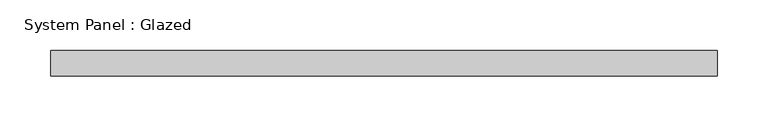
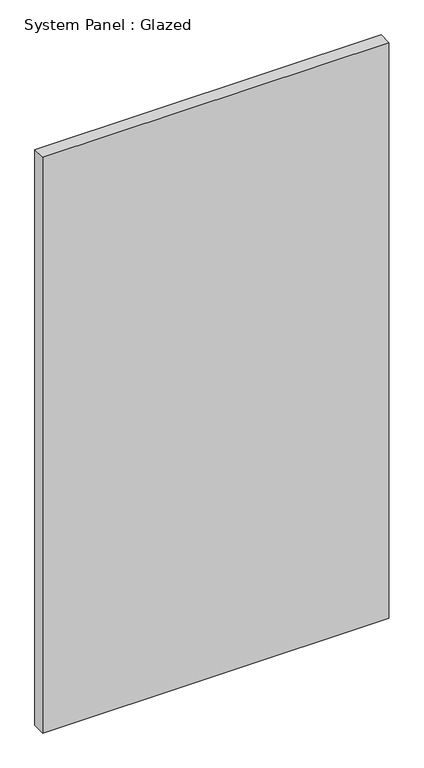
"""IFC4 building model written with IfcOpenShell, lengths in millimetres: plate geometry, System Panel : Glazed."""

from ifc_helpers import new_model, si_unit, origin, origin_with_axes, place, context, project, spatial, polyline, outline, extrude, source, transform, mapped, element, save


def system_panel_glazed_c4418efd(model_context):
    return source(origin(), model_context, "Body", "SweptSolid", [
        extrude(outline(polyline([(328.55491, 19.05), (-328.55491, 19.05), (-328.55491, 44.45), (328.55491, 44.45), (328.55491, 19.05)])), origin_with_axes(), (0.0, 0.0, 1.0), 1155.7),
    ])


if __name__ == "__main__":
    model = new_model("IFC4")
    model_context = context("Model", 3, world=origin())
    ifc_project = project(units=[si_unit("LENGTHUNIT", "METRE", prefix="MILLI")], contexts=[model_context])
    site = spatial("IfcSite", under=ifc_project)
    building = spatial("IfcBuilding", under=site)
    placement = place(None, origin())
    system_panel_glazed_shape = system_panel_glazed_c4418efd(model_context)
    element("IfcPlate", 1, ObjectType="System Panel : Glazed", at=placement, inside=building, context=model_context, shape_type="MappedRepresentation", body=[
        mapped(system_panel_glazed_shape, transform((0.0, 0.0, 0.0), x_axis=(1.0, 0.0, 0.0), y_axis=(0.0, 1.0, 0.0), z_axis=(0.0, 0.0, 1.0))),
    ])
    save(model, "model.ifc")

# Revit data of these elements
# Type "System Panel : Glazed"
#   Construction Type Id = "GSP4R"
#   Analytic Construction = "1/8 in Pilkington single glazing"
#   Visual Light Transmittance = 0.9
#   Solar Heat Gain Coefficient = 0.86
#   Heat Transfer Coefficient (U) = 1.18115 BTU/(h·ft²·°F)
# Element 1 (IfcPlate, "System Panel : Glazed")
#   Materials on its faces: "Glass"
# Materials
#   "Glass": class "Glass", colour RGB 0 128 192, transparency 0.75, Description = "Soda Lime Glass", Cost = 0
